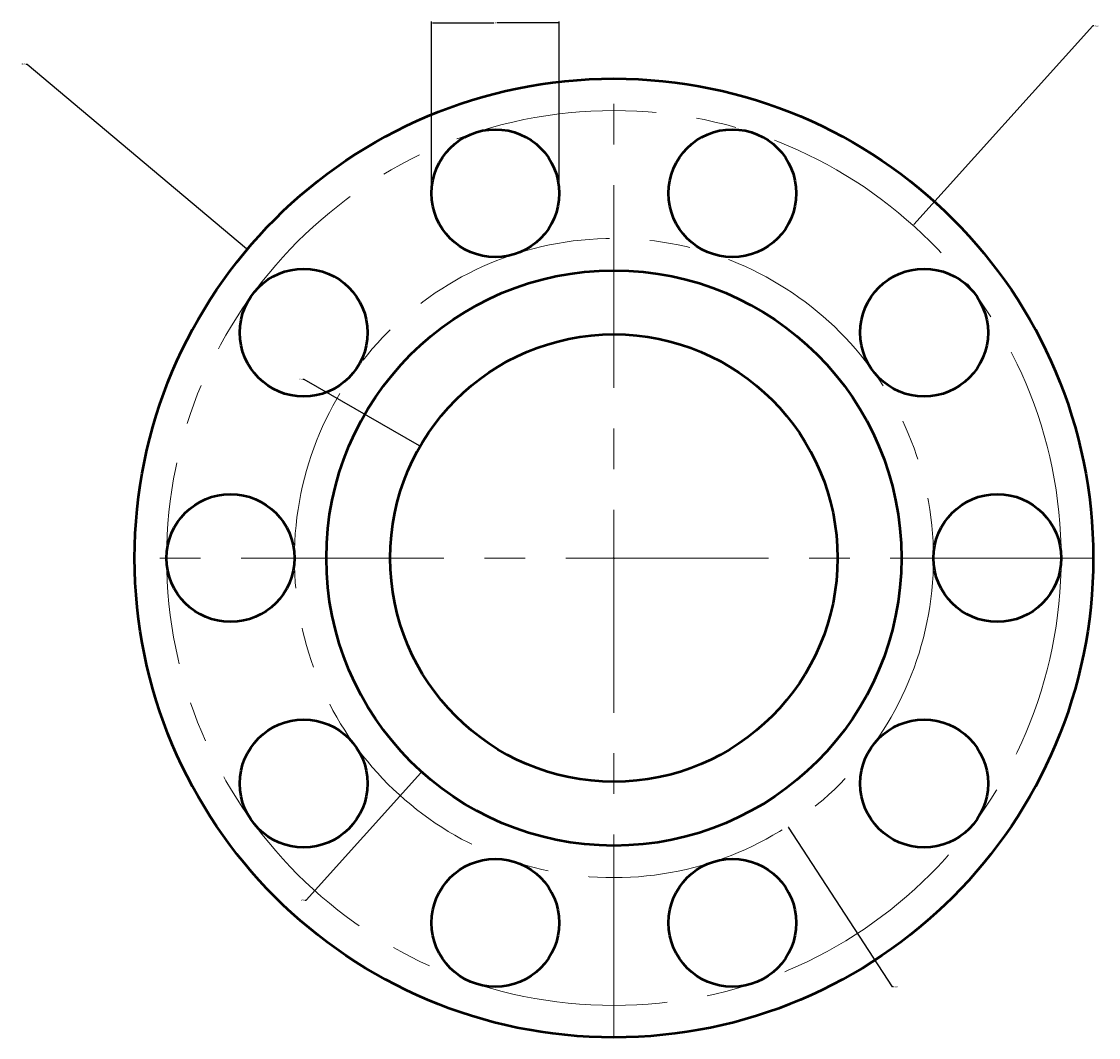
# Model space of a CAD drawing. Units: millimetres. Extents: x 80 to 248, y 56 to 215.
import ezdxf

# ---------------------------------------------------------------- set-up
doc = ezdxf.new("R2010")
doc.units = ezdxf.units.MM
doc.linetypes.add('CENTER', pattern=[50.8, 31.75, -6.35, 6.35, -6.35])
for name, color, linetype, lineweight in [('M-CNTR', 7, 'CENTER', 18), ('M-DIMS', 2, 'Continuous', 18), ('M-OUTL', 7, 'Continuous', 50)]:
    doc.layers.add(name, color=color, linetype=linetype, lineweight=lineweight)
doc.styles.get("Standard").update_dxf_attribs({"font": 'arial.ttf'})
doc.dimstyles.get("Standard").update_dxf_attribs({"dimtxt": 0.18, "dimasz": 0.18, "dimexe": 0.18, "dimexo": 0.0625, "dimgap": 0.09, "dimtad": 0, "dimtih": 1, "dimtoh": 1, "dimdec": 4, "dimzin": 0, "dimdsep": 46, "dimtxsty": 'Standard', "dimcen": 0.09, "dimadec": 0, "dimazin": 0, "dimtfac": 1, "dimtdec": 4, "dimtofl": 0, "dimtmove": 0, "dimatfit": 3, "dimfxl": 1, "dimtolj": 1, "dimtzin": 0, "dimarcsym": 0})

# ---------------------------------------------------------------- blocks, each defined once
blk = doc.blocks.new('*U1')
blk.add_circle((0, 0), 10)
blk = doc.blocks.new('*U2')
at = {"layer": 'M-OUTL', "color": 0, "linetype": 'ByBlock', "lineweight": -2, "transparency": 16777216}
for p, rotation in [((153.82, 117.83), 288), ((190.91, 117.83), 252), ((123.82, 96.03), 324), ((220.91, 96.03), 216), ((232.37, 60.77), 180), ((123.82, 25.5), 36.00000000000008), ((220.91, 25.5), 144), ((153.82, 3.7), 72.00000000000006), ((190.91, 3.7), 108)]:
    blk.add_blockref('*U1', p, dxfattribs=dict(at, rotation=rotation))
blk.add_blockref('*U1', (112.37, 60.77), dxfattribs=at)
blk = doc.blocks.new('*D3')
at = {"layer": 'Defpoints', "color": 0, "transparency": 16777216}
for p in [(163.82, 214.52), (143.82, 187.83), (163.82, 187.83)]:
    blk.add_point(p, dxfattribs=at)
at = {"layer": 'M-DIMS', "color": 0, "lineweight": -2, "transparency": 16777216}
for p, q in [((143.82, 187.89), (143.82, 214.7)), ((144, 214.52), (153.6, 214.52)), ((163.64, 214.52), (154.04, 214.52)), ((163.82, 187.89), (163.82, 214.7))]:
    blk.add_line(p, q, dxfattribs=at)
at = {"layer": 'M-DIMS', "color": 0, "transparency": 16777216}
for points in [[(144, 214.55), (144, 214.49), (143.82, 214.52)], [(163.64, 214.55), (163.64, 214.49), (163.82, 214.52)]]:
    blk.add_solid(points, dxfattribs=at)
at = {"layer": 'M-DIMS', "color": 0, "transparency": 16777216, "insert": (153.82, 214.52), "char_height": 0.18, "attachment_point": 5}
blk.add_mtext('\\A1;20', dxfattribs=at)
blk = doc.blocks.new('*D4')
at = {"layer": 'Defpoints', "color": 0, "transparency": 16777216}
for p in [(114.99, 179.07), (229.74, 82.46)]:
    blk.add_point(p, dxfattribs=at)
at = {"layer": 'M-DIMS', "color": 0, "lineweight": -2, "transparency": 16777216}
for p, q in [((80.38, 208.05), (80.56, 208.05)), ((80.56, 208.05), (114.85, 179.18)), ((172.28, 130.77), (172.46, 130.77)), ((172.37, 130.68), (172.37, 130.86))]:
    blk.add_line(p, q, dxfattribs=at)
at = {"layer": 'M-DIMS', "color": 0, "transparency": 16777216}
blk.add_solid([(114.87, 179.21), (114.83, 179.16), (114.99, 179.07)], dxfattribs=at)
at = {"layer": 'M-DIMS', "color": 0, "transparency": 16777216, "insert": (80, 208.05), "char_height": 0.18, "attachment_point": 5}
blk.add_mtext('\\A1;∅150', dxfattribs=at)
blk = doc.blocks.new('*D5')
at = {"layer": 'Defpoints', "color": 0, "transparency": 16777216}
for p in [(219.2, 182.79), (125.53, 78.74)]:
    blk.add_point(p, dxfattribs=at)
at = {"layer": 'M-DIMS', "color": 0, "lineweight": -2, "transparency": 16777216}
for p, q in [((247.3, 214), (219.32, 182.92)), ((247.48, 214), (247.3, 214)), ((172.28, 130.77), (172.46, 130.77)), ((172.37, 130.68), (172.37, 130.86))]:
    blk.add_line(p, q, dxfattribs=at)
at = {"layer": 'M-DIMS', "color": 0, "transparency": 16777216}
blk.add_solid([(219.3, 182.94), (219.34, 182.9), (219.2, 182.79)], dxfattribs=at)
at = {"layer": 'M-DIMS', "color": 0, "transparency": 16777216, "insert": (247.87, 214), "char_height": 0.18, "attachment_point": 5}
blk.add_mtext('\\A1;∅140', dxfattribs=at)
blk = doc.blocks.new('*D6')
at = {"layer": 'Defpoints', "color": 0, "transparency": 16777216}
for p in [(145.13, 172.7), (199.6, 88.83)]:
    blk.add_point(p, dxfattribs=at)
at = {"layer": 'M-DIMS', "color": 0, "lineweight": -2, "transparency": 16777216}
for p, q in [((172.28, 130.77), (172.46, 130.77)), ((172.37, 130.68), (172.37, 130.86)), ((215.94, 63.67), (199.7, 88.68)), ((216.12, 63.67), (215.94, 63.67))]:
    blk.add_line(p, q, dxfattribs=at)
at = {"layer": 'M-DIMS', "color": 0, "transparency": 16777216}
blk.add_solid([(199.72, 88.7), (199.67, 88.67), (199.6, 88.83)], dxfattribs=at)
at = {"layer": 'M-DIMS', "color": 0, "transparency": 16777216, "insert": (216.5, 63.67), "char_height": 0.18, "attachment_point": 5}
blk.add_mtext('\\A1;∅100', dxfattribs=at)
blk = doc.blocks.new('*D7')
at = {"layer": 'Defpoints', "color": 0, "transparency": 16777216}
for p in [(202.48, 164.21), (142.25, 97.33)]:
    blk.add_point(p, dxfattribs=at)
at = {"layer": 'M-DIMS', "color": 0, "lineweight": -2, "transparency": 16777216}
for p, q in [((172.28, 130.77), (172.46, 130.77)), ((172.37, 130.68), (172.37, 130.86)), ((124.19, 77.26), (142.13, 97.19)), ((124.01, 77.26), (124.19, 77.26))]:
    blk.add_line(p, q, dxfattribs=at)
at = {"layer": 'M-DIMS', "color": 0, "transparency": 16777216}
blk.add_solid([(142.11, 97.21), (142.16, 97.17), (142.25, 97.33)], dxfattribs=at)
at = {"layer": 'M-DIMS', "color": 0, "transparency": 16777216, "insert": (123.69, 77.26), "char_height": 0.18, "attachment_point": 5}
blk.add_mtext('\\A1;∅90', dxfattribs=at)
blk = doc.blocks.new('*D8')
at = {"layer": 'Defpoints', "color": 0, "transparency": 16777216}
for p in [(142.05, 148.26), (202.68, 113.27)]:
    blk.add_point(p, dxfattribs=at)
at = {"layer": 'M-DIMS', "color": 0, "lineweight": -2, "transparency": 16777216}
for p, q in [((123.68, 158.76), (123.86, 158.76)), ((123.86, 158.76), (141.89, 148.35)), ((172.28, 130.77), (172.46, 130.77)), ((172.37, 130.68), (172.37, 130.86))]:
    blk.add_line(p, q, dxfattribs=at)
at = {"layer": 'M-DIMS', "color": 0, "transparency": 16777216}
blk.add_solid([(141.91, 148.38), (141.88, 148.32), (142.05, 148.26)], dxfattribs=at)
at = {"layer": 'M-DIMS', "color": 0, "transparency": 16777216, "insert": (123.37, 158.76), "char_height": 0.18, "attachment_point": 5}
blk.add_mtext('\\A1;∅70', dxfattribs=at)

msp = doc.modelspace()

# ---------------------------------------------------------------- linework, layer by layer
at = {"layer": 'M-CNTR'}
for p, q in [((172.37, 55.77), (172.37, 205.77)), ((247.37, 130.77), (97.37, 130.77)), ((172.37, 130.77), (172.37, 130.77))]:
    msp.add_line(p, q, dxfattribs=at)
for radius in [70, 50]:
    msp.add_circle((172.37, 130.77), radius, dxfattribs=at)
at = {"layer": 'M-OUTL'}
for radius in [75, 45, 35]:
    msp.add_circle((172.37, 130.77), radius, dxfattribs=at)

# ---------------------------------------------------------------- block references
msp.add_blockref('*U2', (0, 70), dxfattribs=at)

# ---------------------------------------------------------------- dimensions: what is measured, and where the dimension line sits
at = {"layer": 'M-DIMS'}
for p1, p2, picture, middle in [((125.53, 78.74), (219.2, 182.79), '*D5', (247.87, 214)), ((229.74, 82.46), (114.99, 179.07), '*D4', (80, 208.05)), ((145.13, 172.7), (199.6, 88.83), '*D6', (216.5, 63.67)), ((202.48, 164.21), (142.25, 97.33), '*D7', (123.69, 77.26)), ((202.68, 113.27), (142.05, 148.26), '*D8', (123.37, 158.76))]:
    dim = msp.add_diameter_dim_2p(p1=p1, p2=p2, dimstyle='Standard', override={"dimdec": 0, "dimlfac": 1, "dimrnd": 0, "dimzin": 0, "dimdsep": 46, "dimlunit": 2}, dxfattribs=at)
    dim.commit()
    dim.dimension.update_dxf_attribs({"geometry": picture, "text_midpoint": middle, "dimtype": 163})
dim = msp.add_linear_dim(base=(163.82, 214.52), p1=(143.82, 187.83), p2=(163.82, 187.83), dimstyle='Standard', override={"dimdec": 0, "dimlfac": 1, "dimrnd": 0, "dimzin": 0, "dimdsep": 46, "dimlunit": 2}, dxfattribs=at)
dim.commit()
dim.dimension.update_dxf_attribs({"geometry": '*D3', "text_midpoint": (153.82, 214.52)})

doc.saveas('drawing.dxf')
